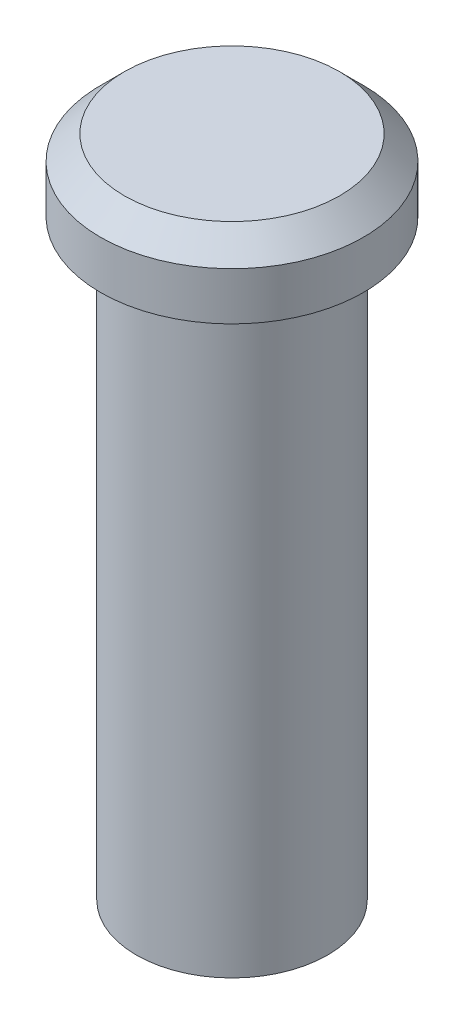
ISO-10303-21;
HEADER;
FILE_DESCRIPTION(('STEP AP214'),'2;1');
FILE_NAME('part.step','',(''),(''),'','','');
FILE_SCHEMA(('AUTOMOTIVE_DESIGN { 1 0 10303 214 1 1 1 1 }'));
ENDSEC;
DATA;
#1=APPLICATION_CONTEXT('core data for automotive mechanical design processes');
#2=APPLICATION_PROTOCOL_DEFINITION('international standard','automotive_design',2000,#1);
#3=PRODUCT_CONTEXT('',#1,'mechanical');
#4=PRODUCT('Part','Part','',(#3));
#5=PRODUCT_RELATED_PRODUCT_CATEGORY('part','',(#4));
#6=PRODUCT_DEFINITION_FORMATION('','',#4);
#7=PRODUCT_DEFINITION_CONTEXT('part definition',#1,'design');
#8=PRODUCT_DEFINITION('design','',#6,#7);
#9=PRODUCT_DEFINITION_SHAPE('','',#8);
#10=(LENGTH_UNIT() NAMED_UNIT(*) SI_UNIT(.MILLI.,.METRE.));
#11=(NAMED_UNIT(*) PLANE_ANGLE_UNIT() SI_UNIT($,.RADIAN.));
#12=(NAMED_UNIT(*) SI_UNIT($,.STERADIAN.) SOLID_ANGLE_UNIT());
#13=UNCERTAINTY_MEASURE_WITH_UNIT(LENGTH_MEASURE(1.E-05),#10,'distance_accuracy_value','');
#14=(GEOMETRIC_REPRESENTATION_CONTEXT(3) GLOBAL_UNCERTAINTY_ASSIGNED_CONTEXT((#13)) GLOBAL_UNIT_ASSIGNED_CONTEXT((#10,
#11,#12)) REPRESENTATION_CONTEXT('',''));
#15=CARTESIAN_POINT('',(0.,0.,0.));
#16=DIRECTION('',(0.,0.,1.));
#17=DIRECTION('',(1.,0.,0.));
#18=AXIS2_PLACEMENT_3D('',#15,#16,#17);
#19=CARTESIAN_POINT('',(0.,24.75,0.));
#20=DIRECTION('',(0.,-1.,0.));
#21=DIRECTION('',(0.,0.,-1.));
#22=AXIS2_PLACEMENT_3D('',#19,#20,#21);
#23=CYLINDRICAL_SURFACE('',#22,4.);
#24=CARTESIAN_POINT('',(0.,24.75,0.));
#25=DIRECTION('',(0.,1.,0.));
#26=DIRECTION('',(0.,0.,1.));
#27=AXIS2_PLACEMENT_3D('',#24,#25,#26);
#28=CIRCLE('',#27,4.);
#29=CARTESIAN_POINT('',(0.,24.75,4.));
#30=VERTEX_POINT('',#29);
#31=EDGE_CURVE('E52',#30,#30,#28,.T.);
#32=ORIENTED_EDGE('',*,*,#31,.F.);
#33=EDGE_LOOP('',(#32));
#34=FACE_BOUND('',#33,.T.);
#35=CARTESIAN_POINT('',(0.,0.,0.));
#36=DIRECTION('',(0.,1.,0.));
#37=DIRECTION('',(0.,0.,1.));
#38=AXIS2_PLACEMENT_3D('',#35,#36,#37);
#39=CIRCLE('',#38,4.);
#40=CARTESIAN_POINT('',(0.,0.,4.));
#41=VERTEX_POINT('',#40);
#42=EDGE_CURVE('E60',#41,#41,#39,.T.);
#43=ORIENTED_EDGE('',*,*,#42,.T.);
#44=EDGE_LOOP('',(#43));
#45=FACE_BOUND('',#44,.T.);
#46=ADVANCED_FACE('F41',(#34,#45),#23,.T.);
#47=CARTESIAN_POINT('',(0.,0.,0.));
#48=DIRECTION('',(0.,1.,0.));
#49=DIRECTION('',(0.,0.,1.));
#50=AXIS2_PLACEMENT_3D('',#47,#48,#49);
#51=PLANE('',#50);
#52=ORIENTED_EDGE('',*,*,#42,.F.);
#53=EDGE_LOOP('',(#52));
#54=FACE_BOUND('',#53,.T.);
#55=ADVANCED_FACE('F85',(#54),#51,.F.);
#56=CARTESIAN_POINT('',(0.,27.75,0.));
#57=DIRECTION('',(0.,-1.,0.));
#58=DIRECTION('',(0.,0.,-1.));
#59=AXIS2_PLACEMENT_3D('',#56,#57,#58);
#60=CYLINDRICAL_SURFACE('',#59,5.5);
#61=CARTESIAN_POINT('',(0.,26.75,0.));
#62=DIRECTION('',(0.,1.,0.));
#63=DIRECTION('',(0.,0.,1.));
#64=AXIS2_PLACEMENT_3D('',#61,#62,#63);
#65=CIRCLE('',#64,5.5);
#66=CARTESIAN_POINT('',(0.,26.75,5.5));
#67=VERTEX_POINT('',#66);
#68=EDGE_CURVE('E10',#67,#67,#65,.F.);
#69=ORIENTED_EDGE('',*,*,#68,.T.);
#70=EDGE_LOOP('',(#69));
#71=FACE_BOUND('',#70,.T.);
#72=CARTESIAN_POINT('',(0.,24.75,0.));
#73=DIRECTION('',(0.,1.,0.));
#74=DIRECTION('',(0.,0.,1.));
#75=AXIS2_PLACEMENT_3D('',#72,#73,#74);
#76=CIRCLE('',#75,5.5);
#77=CARTESIAN_POINT('',(0.,24.75,5.5));
#78=VERTEX_POINT('',#77);
#79=EDGE_CURVE('E61',#78,#78,#76,.T.);
#80=ORIENTED_EDGE('',*,*,#79,.T.);
#81=EDGE_LOOP('',(#80));
#82=FACE_BOUND('',#81,.T.);
#83=ADVANCED_FACE('F67',(#71,#82),#60,.T.);
#84=CARTESIAN_POINT('',(0.,27.75,0.));
#85=DIRECTION('',(0.,1.,0.));
#86=DIRECTION('',(0.,0.,1.));
#87=AXIS2_PLACEMENT_3D('',#84,#85,#86);
#88=PLANE('',#87);
#89=CARTESIAN_POINT('',(0.,27.75,0.));
#90=DIRECTION('',(0.,1.,0.));
#91=DIRECTION('',(0.,0.,1.));
#92=AXIS2_PLACEMENT_3D('',#89,#90,#91);
#93=CIRCLE('',#92,4.5);
#94=CARTESIAN_POINT('',(0.,27.75,4.5));
#95=VERTEX_POINT('',#94);
#96=EDGE_CURVE('E47',#95,#95,#93,.T.);
#97=ORIENTED_EDGE('',*,*,#96,.T.);
#98=EDGE_LOOP('',(#97));
#99=FACE_BOUND('',#98,.T.);
#100=ADVANCED_FACE('F68',(#99),#88,.T.);
#101=CARTESIAN_POINT('',(0.,24.75,0.));
#102=DIRECTION('',(0.,1.,0.));
#103=DIRECTION('',(0.,0.,1.));
#104=AXIS2_PLACEMENT_3D('',#101,#102,#103);
#105=PLANE('',#104);
#106=ORIENTED_EDGE('',*,*,#31,.T.);
#107=EDGE_LOOP('',(#106));
#108=FACE_BOUND('',#107,.T.);
#109=ORIENTED_EDGE('',*,*,#79,.F.);
#110=EDGE_LOOP('',(#109));
#111=FACE_BOUND('',#110,.T.);
#112=ADVANCED_FACE('F70',(#108,#111),#105,.F.);
#113=CARTESIAN_POINT('',(0.,27.75,0.));
#114=DIRECTION('',(0.,-1.,0.));
#115=DIRECTION('',(0.,0.,-1.));
#116=AXIS2_PLACEMENT_3D('',#113,#114,#115);
#117=CONICAL_SURFACE('',#116,4.5,0.785398163397447);
#118=ORIENTED_EDGE('',*,*,#68,.F.);
#119=EDGE_LOOP('',(#118));
#120=FACE_BOUND('',#119,.T.);
#121=ORIENTED_EDGE('',*,*,#96,.F.);
#122=EDGE_LOOP('',(#121));
#123=FACE_BOUND('',#122,.T.);
#124=ADVANCED_FACE('F42',(#120,#123),#117,.T.);
#125=CLOSED_SHELL('',(#46,#55,#83,#100,#112,#124));
#126=MANIFOLD_SOLID_BREP('B2',#125);
#127=ADVANCED_BREP_SHAPE_REPRESENTATION('',(#18,#126),#14);
#128=SHAPE_DEFINITION_REPRESENTATION(#9,#127);
ENDSEC;
END-ISO-10303-21;
